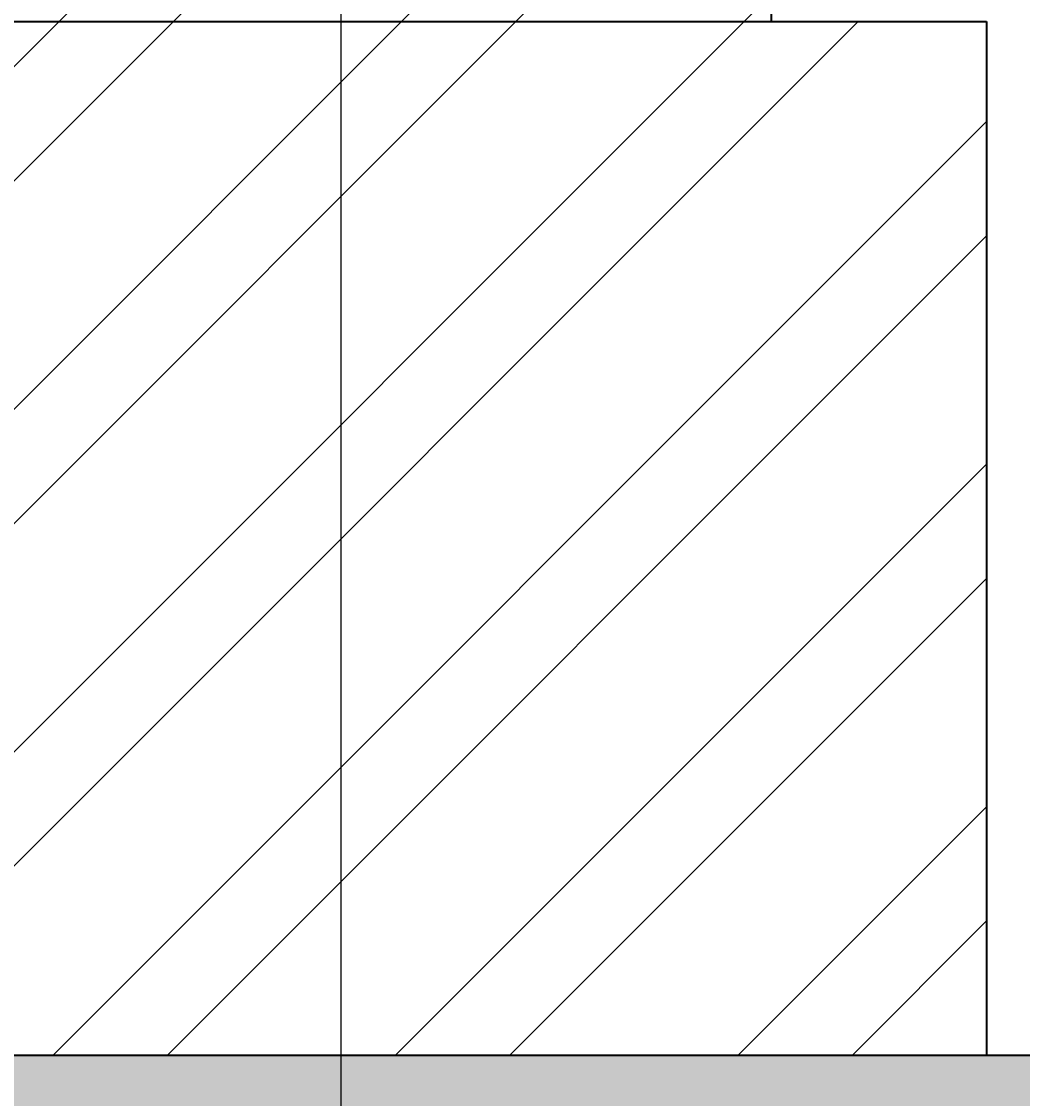
# Model space of a CAD drawing. Units: inches. Extents: x -301 to 715, y -607 to 364.
# Tile 6 of 141: x -43 to -19, y -536 to -511. Entities that reach past the tile are written whole.
import ezdxf

# ---------------------------------------------------------------- set-up
doc = ezdxf.new("R2010")
doc.units = ezdxf.units.IN
doc.header["$MEASUREMENT"] = 0
for name, color, linetype, lineweight in [('A-ANNO-DIMS', 2, 'Continuous', 18), ('A-SECT-PATT', 8, 'Continuous', 13), ('S-FNDN', 2, 'Continuous', 35)]:
    doc.layers.add(name, color=color, linetype=linetype, lineweight=lineweight)
doc.styles.get("Standard").update_dxf_attribs({"font": 'arial.ttf'})
doc.dimstyles.get("Standard").update_dxf_attribs({"dimtxt": 0.18, "dimasz": 0.18, "dimexe": 0.18, "dimexo": 0.0625, "dimgap": 0.09, "dimtad": 0, "dimtih": 1, "dimtoh": 1, "dimdec": 1, "dimzin": 0, "dimdsep": 46, "dimlunit": 4, "dimtxsty": 'Standard', "dimcen": 0.09, "dimclrd": 3, "dimclre": 4, "dimclrt": 6, "dimadec": 0, "dimazin": 0, "dimtfac": 1, "dimtdec": 1, "dimtofl": 0, "dimtmove": 0, "dimatfit": 3, "dimfxl": 1, "dimtfill": 2, "dimtfillclr": 51, "dimtolj": 1, "dimtzin": 0, "dimarcsym": 0})

# ---------------------------------------------------------------- blocks, each defined once
blk = doc.blocks.new('*D179')
at = {"layer": 'A-ANNO-DIMS', "color": 4, "lineweight": -2, "transparency": 16777216}
for p, q in [((-87.981, -433.54), (-87.981, -573.809)), ((-35.282, -463.54), (-35.282, -573.809))]:
    blk.add_line(p, q, dxfattribs=at)
at = {"layer": 'A-ANNO-DIMS', "color": 3, "lineweight": -2, "transparency": 16777216}
for p, q in [((-87.801, -573.629), (-62.174, -573.629)), ((-35.462, -573.629), (-61.089, -573.629))]:
    blk.add_line(p, q, dxfattribs=at)
at = {"layer": 'A-ANNO-DIMS', "color": 3, "transparency": 16777216}
for points in [[(-87.801, -573.599), (-87.801, -573.659), (-87.981, -573.629)], [(-35.462, -573.599), (-35.462, -573.659), (-35.282, -573.629)]]:
    blk.add_solid(points, dxfattribs=at)
at = {"layer": 'Defpoints', "color": 0, "transparency": 16777216}
for p in [(-87.981, -433.477), (-35.282, -463.477), (-35.282, -573.629)]:
    blk.add_point(p, dxfattribs=at)
at = {"layer": 'A-ANNO-DIMS', "color": 6, "transparency": 16777216, "insert": (-61.631, -573.629), "char_height": 0.18, "attachment_point": 5, "bg_fill": 1, "box_fill_scale": 1.25, "bg_fill_color": 51, "bg_fill_transparency": 0}
blk.add_mtext('\\A1;4\'-4 1/2"', dxfattribs=at)
blk = doc.blocks.new('*D180')
at = {"layer": 'A-ANNO-DIMS', "color": 4, "lineweight": -2, "transparency": 16777216}
for p, q in [((-35.282, -463.54), (-35.282, -573.809)), ((12.718, -463.54), (12.718, -573.809))]:
    blk.add_line(p, q, dxfattribs=at)
at = {"layer": 'A-ANNO-DIMS', "color": 3, "lineweight": -2, "transparency": 16777216}
for p, q in [((-35.102, -573.629), (-11.615, -573.629)), ((12.538, -573.629), (-10.949, -573.629))]:
    blk.add_line(p, q, dxfattribs=at)
at = {"layer": 'A-ANNO-DIMS', "color": 3, "transparency": 16777216}
for points in [[(-35.102, -573.599), (-35.102, -573.659), (-35.282, -573.629)], [(12.538, -573.599), (12.538, -573.659), (12.718, -573.629)]]:
    blk.add_solid(points, dxfattribs=at)
at = {"layer": 'Defpoints', "color": 0, "transparency": 16777216}
for p in [(-35.282, -463.477), (12.718, -463.477), (12.718, -573.629)]:
    blk.add_point(p, dxfattribs=at)
at = {"layer": 'A-ANNO-DIMS', "color": 6, "transparency": 16777216, "insert": (-11.282, -573.629), "char_height": 0.18, "attachment_point": 5, "bg_fill": 1, "box_fill_scale": 1.25, "bg_fill_color": 51, "bg_fill_transparency": 0}
blk.add_mtext('\\A1;4\'-0"', dxfattribs=at)
blk = doc.blocks.new('*D191')
at = {"layer": 'A-ANNO-DIMS', "color": 4, "lineweight": -2, "transparency": 16777216}
for p, q in [((129.193, -481.477), (-266.112, -481.477)), ((114.193, -540.477), (-266.112, -540.477))]:
    blk.add_line(p, q, dxfattribs=at)
at = {"layer": 'A-ANNO-DIMS', "color": 3, "lineweight": -2, "transparency": 16777216}
for p, q in [((-265.932, -481.657), (-265.932, -510.797)), ((-265.932, -540.297), (-265.932, -511.158))]:
    blk.add_line(p, q, dxfattribs=at)
at = {"layer": 'A-ANNO-DIMS', "color": 3, "transparency": 16777216}
for points in [[(-265.962, -481.657), (-265.902, -481.657), (-265.932, -481.477)], [(-265.962, -540.297), (-265.902, -540.297), (-265.932, -540.477)]]:
    blk.add_solid(points, dxfattribs=at)
at = {"layer": 'Defpoints', "color": 0, "transparency": 16777216}
for p in [(129.255, -481.477), (-265.932, -540.477), (114.255, -540.477)]:
    blk.add_point(p, dxfattribs=at)
at = {"layer": 'A-ANNO-DIMS', "color": 6, "transparency": 16777216, "insert": (-265.932, -510.977), "char_height": 0.18, "attachment_point": 5, "bg_fill": 1, "box_fill_scale": 1.25, "bg_fill_color": 51, "bg_fill_transparency": 0}
blk.add_mtext('\\A1;4\'-11"', dxfattribs=at)

msp = doc.modelspace()

# ---------------------------------------------------------------- hatches: boundary and pattern name
at = {"layer": 'A-SECT-PATT'}
h = msp.add_hatch(dxfattribs=at)
h.set_pattern_fill('ANSI32', color=256, scale=15)
h.set_pattern_definition([(45, (10.321, 33.8764), (-3.977476, 3.977476), []), (45, (12.973, 33.8764), (-3.977476, 3.977476), [])])
h.paths.add_polyline_path([(-185.282, -324.477), (-199.282, -324.477), (-199.282, -329.477), (-194.282, -329.477), (-194.282, -353.477), (-185.282, -353.477)])
h.paths.add_polyline_path([(-185.282, -361.477), (-193.904, -361.477), (-193.982, -377.537), (-185.282, -377.537)])
h.paths.add_polyline_path([(143.218, -329.477), (148.218, -329.477), (148.218, -324.477), (134.255, -324.477), (134.255, -353.477), (143.218, -353.477)])
h.paths.add_polyline_path([(143.218, -361.477), (134.255, -361.477), (134.255, -377.477), (143.218, -377.477)])
h.paths.add_polyline_path([(-185.282, -439.477), (-194.282, -439.477), (-194.282, -463.477), (-185.282, -463.477)])
h.paths.add_polyline_path([(-185.282, -471.477), (-194.282, -471.477), (-194.282, -481.477), (-185.282, -481.477)])
h.paths.add_polyline_path([(-185.282, -463.477), (-194.282, -463.477), (-194.282, -466.477), (-185.282, -466.477)])
h.paths.add_polyline_path([(-185.282, -466.477), (-194.282, -466.477), (-194.282, -471.477), (-185.282, -471.477)])
h.paths.add_polyline_path([(-180.282, -481.477), (-185.282, -481.477), (-194.282, -481.477), (-199.282, -481.477), (-199.282, -493.477), (-180.282, -493.477)])
h.paths.add_polyline_path([(-175.282, -493.477), (-180.282, -493.477), (-199.282, -493.477), (-204.282, -493.477), (-204.282, -511.477), (-175.282, -511.477)])
h.paths.add_polyline_path([(-170.282, -511.477), (-175.282, -511.477), (-204.282, -511.477), (-209.282, -511.477), (-209.282, -535.477), (-170.282, -535.477)])
h.paths.add_polyline_path([(-35.282, -463.477), (-41.282, -463.477), (-41.282, -466.477), (-35.282, -466.477)])
h.paths.add_polyline_path([(-35.282, -466.477), (-41.282, -466.477), (-41.282, -471.477), (-35.282, -471.477)])
h.paths.add_polyline_path([(-35.282, -471.477), (-41.282, -471.477), (-41.282, -481.477), (-35.282, -481.477)])
h.paths.add_polyline_path([(-30.282, -481.477), (-46.282, -481.477), (-46.282, -493.477), (-30.282, -493.477)])
h.paths.add_polyline_path([(-25.282, -493.477), (-30.282, -493.477), (-46.282, -493.477), (-51.282, -493.477), (-51.282, -511.477), (-25.282, -511.477)])
h.paths.add_polyline_path([(-20.282, -511.477), (-25.282, -511.477), (-51.282, -511.477), (-56.282, -511.477), (-56.282, -535.477), (-20.282, -535.477)])
h.paths.add_polyline_path([(143.218, -463.477), (134.255, -463.477), (134.255, -466.477), (143.218, -466.477)])
h.paths.add_polyline_path([(143.218, -466.477), (134.255, -466.477), (134.255, -471.477), (143.218, -471.477)])
h.paths.add_polyline_path([(143.218, -471.477), (134.255, -471.477), (134.255, -481.477), (143.218, -481.477)])
h.paths.add_polyline_path([(148.255, -481.477), (143.255, -481.477), (134.255, -481.477), (129.255, -481.477), (129.255, -493.477), (148.255, -493.477)])
h.paths.add_polyline_path([(153.255, -493.477), (148.255, -493.477), (129.255, -493.477), (124.255, -493.477), (124.255, -511.477), (153.255, -511.477)])
h.paths.add_polyline_path([(158.255, -511.477), (153.255, -511.477), (124.255, -511.477), (119.255, -511.477), (119.255, -535.477), (158.255, -535.477)])
h = msp.add_hatch(dxfattribs=at)
h.set_pattern_fill('AR-CONC', color=256, scale=0.5)
h.set_pattern_definition([(50, (10.3213, 33.8764), (3.586301, -0.31376), [0.375, -4.125]), (355, (10.3213, 33.8764), (-0.693757, 3.76096), [0.3, -3.3]), (100.45144, (10.62, 33.8502), (2.892544, 3.4472), [0.3187, -3.50571]), (46.1842, (10.3213, 34.8764), (5.336207, -0.827596), [0.5625, -6.1875]), (96.6356, (10.766, 34.8074), (4.67331, 4.870593), [0.47805, -5.25857]), (351.1842, (10.321, 34.8764), (4.67331, 4.870593), [0.45, -4.95]), (21, (10.8213, 34.6264), (2.984535, -2.013094), [0.375, -4.125]), (326, (10.8213, 34.6264), (1.216577, 3.62575), [0.3, -3.3]), (71.45144, (11.07, 34.4586), (4.201112, 1.612656), [0.3187, -3.50571]), (37.5, (10.3213, 33.8764), (0.0607993, 1.6644693), [0, -3.26, 0, -3.35, 0, -3.3125]), (7.5, (10.3213, 33.8764), (1.3153477, 1.9720586), [0, -1.91, 0, -3.185, 0, -1.2625]), (327.5, (9.2063, 33.8764), (2.6691122, -0.1127744), [0, -1.25, 0, -3.9, 0, -5.175]), (317.5, (8.7063, 33.8764), (2.915931, 0.500525), [0, -1.625, 0, -2.59, 0, -3.675])])
h.paths.add_polyline_path([(-56.282, -535.477), (-61.282, -535.477), (-61.282, -540.477), (-15.282, -540.477), (-15.282, -535.477), (-20.282, -535.477)])
h.paths.add_polyline_path([(119.255, -535.477), (114.255, -535.477), (114.255, -540.477), (163.255, -540.477), (163.255, -535.477), (158.255, -535.477)])
h.paths.add_polyline_path([(-206.282, -471.477), (-209.282, -471.477), (-209.282, -481.477), (-206.282, -481.477), (-194.282, -481.477), (-194.282, -471.477)])
h.paths.add_polyline_path([(-41.282, -481.477), (-41.282, -471.477), (-185.282, -471.477), (-185.282, -481.477), (-180.282, -481.477)])
h.paths.add_polyline_path([(134.255, -481.477), (134.255, -471.477), (-35.282, -471.477), (-35.282, -481.477), (-30.282, -481.477)])
h.paths.add_polyline_path([(155.218, -481.477), (158.218, -481.477), (158.218, -471.477), (153.218, -471.477), (143.218, -471.477), (143.218, -481.477), (148.255, -481.477)])
h.paths.add_polyline_path([(-193.88, -356.477), (-193.904, -361.477), (143.218, -361.477), (143.218, -356.477)])

# ---------------------------------------------------------------- linework, layer by layer
at = {"layer": 'S-FNDN'}
for p, q in [((-25.282, -493.477), (-25.282, -511.477)), ((-51.282, -511.477), (-25.282, -511.477)), ((-25.282, -511.477), (-20.282, -511.477)), ((-20.282, -511.477), (-20.282, -535.477)), ((-56.282, -535.477), (-20.282, -535.477)), ((-20.282, -535.477), (-15.282, -535.477))]:
    msp.add_line(p, q, dxfattribs=at)

# ---------------------------------------------------------------- dimensions: what is measured, and where the dimension line sits
at = {"layer": 'A-ANNO-DIMS'}
for base, p1, p2, picture, middle in [((-35.282, -573.629), (-87.981, -433.477), (-35.282, -463.477), '*D179', (-61.631, -573.629)), ((12.718, -573.629), (-35.282, -463.477), (12.718, -463.477), '*D180', (-11.282, -573.629))]:
    dim = msp.add_linear_dim(base=base, p1=p1, p2=p2, dimstyle='Standard', override={"dimdec": 1, "dimlfac": 1, "dimrnd": 0, "dimzin": 1, "dimdsep": 46, "dimlunit": 4, "dimfrac": 2}, dxfattribs=at)
    dim.commit()
    dim.dimension.update_dxf_attribs({"geometry": picture, "text_midpoint": middle})
dim = msp.add_linear_dim(base=(-265.932, -540.477), p1=(129.255, -481.477), p2=(114.255, -540.477), angle=90, dimstyle='Standard', override={"dimdec": 1, "dimlfac": 1, "dimrnd": 0, "dimzin": 1, "dimdsep": 46, "dimlunit": 4, "dimfrac": 2}, dxfattribs=at)
dim.commit()
dim.dimension.update_dxf_attribs({"geometry": '*D191', "text_midpoint": (-265.932, -510.977)})

doc.saveas('drawing.dxf')
